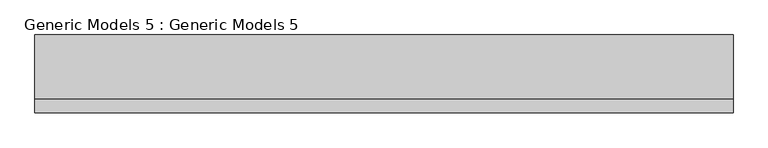
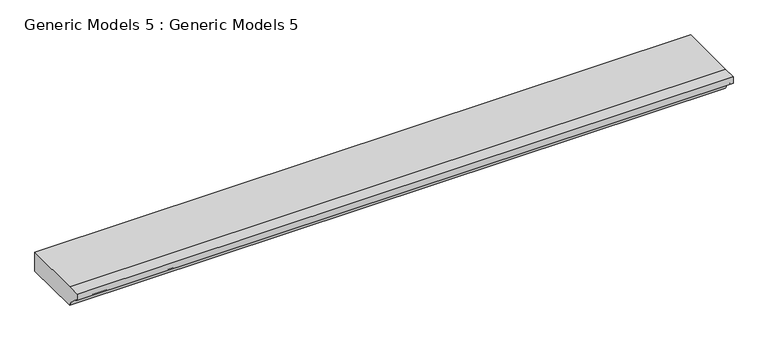
"""IFC4 building model written with IfcOpenShell, lengths in millimetres: proxy geometry, Generic Models 5 : Generic Models 5."""

from ifc_helpers import new_model, si_unit, point, frame, frame_2d, origin, place, context, project, spatial, polyline, circle_curve, trimmed, segment, composite_curve, outline, extrude, source, transform, mapped, element, save


def generic_models_5_generic_models_5_b956d3bb(model_context):
    return source(origin(), model_context, "Body", "SweptSolid", [
        extrude(outline(composite_curve([segment(polyline([(-3431.061407, 7543.8), (-3380.261407, 7543.8), (-3151.661407, 7543.8), (-3151.661407, 7467.6), (-3380.261407, 7467.6)]), True, "CONTINUOUS"), segment(trimmed(circle_curve(frame_2d((-3472.0358422, 7426.6255648)), 100.5059764), [point((-3380.261407, 7467.6))], [point((-3431.061407, 7518.4))], True, "CARTESIAN"), True, "CONTINUOUS"), segment(polyline([(-3431.061407, 7518.4), (-3431.061407, 7543.8)]), True, "CONTINUOUS")], self_intersect=False)), frame((-14902.5371373, 0.0, 0.0), z_axis=(1.0, 0.0, 0.0), x_axis=(0.0, 1.0, 0.0)), (0.0, 0.0, 1.0), 2498.6384509),
    ])


if __name__ == "__main__":
    model = new_model("IFC4")
    model_context = context("Model", 3, world=origin())
    ifc_project = project(units=[si_unit("LENGTHUNIT", "METRE", prefix="MILLI")], contexts=[model_context])
    site = spatial("IfcSite", under=ifc_project)
    building = spatial("IfcBuilding", under=site)
    placement = place(None, origin())
    generic_models_5_generic_models_5_shape = generic_models_5_generic_models_5_b956d3bb(model_context)
    element("IfcBuildingElementProxy", 1, Name="Generic Models 5 : Generic Models 5", ObjectType="Generic Models 5 : Generic Models 5", at=placement, inside=building, context=model_context, shape_type="MappedRepresentation", body=[
        mapped(generic_models_5_generic_models_5_shape, transform((0.0, 0.0, 0.0), x_axis=(1.0, 0.0, 0.0), y_axis=(0.0, 1.0, 0.0), z_axis=(0.0, 0.0, 1.0))),
    ])
    save(model, "model.ifc")
